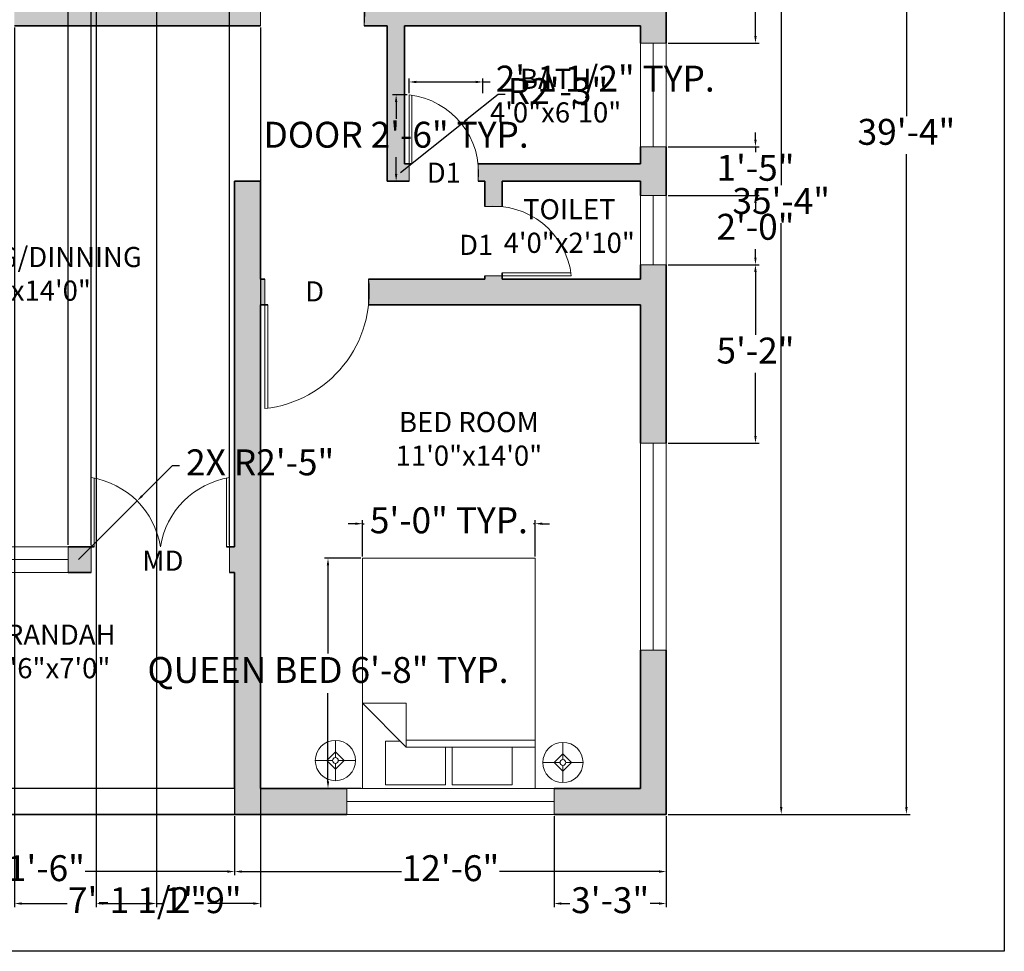
# Model space of a CAD drawing. Units: inches. Extents: x 1942 to 2601, y 2026 to 2623.
# Tile 4 of 5: x 2259 to 2601, y 2026 to 2350. Entities that reach past the tile are written whole.
import ezdxf

# ---------------------------------------------------------------- set-up
doc = ezdxf.new("R2010")
doc.units = ezdxf.units.IN
for name, color, linetype, lineweight in [('A-ANNO-DIMS', 2, 'Continuous', 18), ('A-ANNO-TEXT', 7, 'Continuous', 18), ('A-ANNO-TTLB', 7, 'Continuous', 25), ('A-AREA-IDEN', 7, 'Continuous', 25), ('A-DOOR', 4, 'Continuous', 18), ('A-FLOR', 7, 'Continuous', 25), ('A-FURN', 8, 'Continuous', 18), ('A-GLAZ', 2, 'Continuous', 18), ('A-WALL', 7, 'Continuous', 35), ('A-WALL-PATT', 7, 'Continuous', 13)]:
    doc.layers.add(name, color=color, linetype=linetype, lineweight=lineweight)
doc.styles.get("Standard").update_dxf_attribs({"font": 'arial.ttf'})
doc.dimstyles.new('ISO-25', dxfattribs={"dimtxt": 9, "dimasz": 2.5, "dimexe": 1.25, "dimexo": 0.625, "dimgap": 2, "dimtad": 0, "dimtih": 1, "dimtoh": 1, "dimdec": 1, "dimlunit": 4, "dimtxsty": 'Standard', "dimcen": 2.5, "dimadec": 0, "dimazin": 0, "dimtfac": 0.5, "dimtdec": 1, "dimtmove": 0, "dimatfit": 3, "dimfxl": 1, "dimarcsym": 0})

# ---------------------------------------------------------------- blocks, each defined once
blk = doc.blocks.new('Bed - Queen')
for p, q in [((0, -80.00003), (0, 0)), ((0, 0), (59.99999, 0)), ((59.99999, 0), (59.99999, -80.00003)), ((7.99999, -1.2), (28.79998, -1.2)), ((7.99999, -14.4), (7.99999, -1.2)), ((28.79998, -1.2), (28.79998, -14.4)), ((31.19999, -1.2), (51.99999, -1.2)), ((31.19999, -14.4), (31.19999, -1.2)), ((51.99999, -1.2), (51.99999, -16.4)), ((0, -14.4), (44.8, -14.4)), ((44.8, -16.8), (0, -16.8)), ((59.99999, -29.6), (44.8, -14.4)), ((44.8, -14.4), (44.8, -29.6)), ((51.99999, -16.4), (46.79936, -16.4)), ((44.8, -29.6), (59.99999, -29.6)), ((59.99999, -80.00003), (0, -80.00003))]:
    blk.add_line(p, q)
blk = doc.blocks.new('Lamp - Table')
for p, q in [((0, 7), (0, 1)), ((-1, 0), (-7, 0)), ((0, 3), (-3, 0)), ((-3, 0), (0, -3)), ((3, 0), (0, 3)), ((0, -3), (3, 0)), ((1, 0), (7, 0)), ((0, -1), (0, -7))]:
    blk.add_line(p, q)
for radius in [7, 1]:
    blk.add_circle((0, 0), radius)
blk = doc.blocks.new('*D21')
at = {"layer": 'A-ANNO-DIMS', "color": 0, "lineweight": -2, "transparency": 16777216}
for p, q in [((2195.82, 2073.29), (2195.82, 2052.78)), ((2333.82, 2073.29), (2333.82, 2052.78)), ((2198.32, 2054.03), (2247.78, 2054.03)), ((2331.32, 2054.03), (2281.85, 2054.03))]:
    blk.add_line(p, q, dxfattribs=at)
at = {"layer": 'A-ANNO-DIMS', "color": 0, "transparency": 16777216}
for points in [[(2198.32, 2054.45), (2198.32, 2053.61), (2195.82, 2054.03)], [(2331.32, 2054.45), (2331.32, 2053.61), (2333.82, 2054.03)]]:
    blk.add_solid(points, dxfattribs=at)
at = {"layer": 'Defpoints', "color": 0, "transparency": 16777216}
for p in [(2195.82, 2073.91), (2333.82, 2073.91), (2333.82, 2054.03)]:
    blk.add_point(p, dxfattribs=at)
at = {"layer": 'A-ANNO-DIMS', "color": 0, "transparency": 16777216, "insert": (2264.82, 2054.03), "char_height": 9, "attachment_point": 5}
blk.add_mtext('11\'-6"', dxfattribs=at)
blk = doc.blocks.new('*D22')
at = {"layer": 'A-ANNO-DIMS', "color": 0, "lineweight": -2, "transparency": 16777216}
for p, q in [((2333.82, 2073.29), (2333.82, 2052.78)), ((2483.82, 2073.29), (2483.82, 2052.78)), ((2336.32, 2054.03), (2391.78, 2054.03)), ((2481.32, 2054.03), (2425.85, 2054.03))]:
    blk.add_line(p, q, dxfattribs=at)
at = {"layer": 'A-ANNO-DIMS', "color": 0, "transparency": 16777216}
for points in [[(2336.32, 2054.45), (2336.32, 2053.61), (2333.82, 2054.03)], [(2481.32, 2054.45), (2481.32, 2053.61), (2483.82, 2054.03)]]:
    blk.add_solid(points, dxfattribs=at)
at = {"layer": 'Defpoints', "color": 0, "transparency": 16777216}
for p in [(2333.82, 2073.91), (2483.82, 2073.91), (2483.82, 2054.03)]:
    blk.add_point(p, dxfattribs=at)
at = {"layer": 'A-ANNO-DIMS', "color": 0, "transparency": 16777216, "insert": (2408.82, 2054.03), "char_height": 9, "attachment_point": 5}
blk.add_mtext('12\'-6"', dxfattribs=at)
blk = doc.blocks.new('*D23')
at = {"layer": 'A-ANNO-DIMS', "color": 0, "lineweight": -2, "transparency": 16777216}
for p, q in [((2484.44, 2497.91), (2525.02, 2497.91)), ((2523.77, 2495.41), (2523.77, 2292.51)), ((2523.77, 2076.41), (2523.77, 2279.32)), ((2484.44, 2073.91), (2525.02, 2073.91))]:
    blk.add_line(p, q, dxfattribs=at)
at = {"layer": 'A-ANNO-DIMS', "color": 0, "transparency": 16777216}
for points in [[(2523.35, 2495.41), (2524.19, 2495.41), (2523.77, 2497.91)], [(2523.35, 2076.41), (2524.19, 2076.41), (2523.77, 2073.91)]]:
    blk.add_solid(points, dxfattribs=at)
at = {"layer": 'Defpoints', "color": 0, "transparency": 16777216}
for p in [(2483.82, 2497.91), (2483.82, 2073.91), (2523.77, 2073.91)]:
    blk.add_point(p, dxfattribs=at)
at = {"layer": 'A-ANNO-DIMS', "color": 0, "transparency": 16777216, "insert": (2523.77, 2285.91), "char_height": 9, "attachment_point": 5}
blk.add_mtext('35\'-4"', dxfattribs=at)
blk = doc.blocks.new('*D24')
at = {"layer": 'A-ANNO-DIMS', "color": 0, "lineweight": -2, "transparency": 16777216}
for p, q in [((2484.44, 2545.91), (2568.53, 2545.91)), ((2567.28, 2543.41), (2567.28, 2316.51)), ((2567.28, 2076.41), (2567.28, 2303.32)), ((2484.44, 2073.91), (2568.53, 2073.91))]:
    blk.add_line(p, q, dxfattribs=at)
at = {"layer": 'A-ANNO-DIMS', "color": 0, "transparency": 16777216}
for points in [[(2566.86, 2543.41), (2567.7, 2543.41), (2567.28, 2545.91)], [(2566.86, 2076.41), (2567.7, 2076.41), (2567.28, 2073.91)]]:
    blk.add_solid(points, dxfattribs=at)
at = {"layer": 'Defpoints', "color": 0, "transparency": 16777216}
for p in [(2483.82, 2545.91), (2483.82, 2073.91), (2567.28, 2073.91)]:
    blk.add_point(p, dxfattribs=at)
at = {"layer": 'A-ANNO-DIMS', "color": 0, "transparency": 16777216, "insert": (2567.28, 2309.91), "char_height": 9, "attachment_point": 5}
blk.add_mtext('39\'-4"', dxfattribs=at)
blk = doc.blocks.new('WIN-72IN')
for p, q in [((0, 0), (0, 9)), ((0, 9), (72, 9)), ((72, 0), (72, 9)), ((0, 4.5), (72, 4.5)), ((0, 0), (72, 0))]:
    blk.add_line(p, q)
blk = doc.blocks.new('DOOR-SINGLE-36IN')
for p, q in [((0, 9), (0, 45)), ((1, 9), (1, 44.88)), ((0, 0), (0, 9)), ((36, 0), (36, 9))]:
    blk.add_line(p, q)
blk.add_arc((-4.5, 4.5), 40.75, 353.6598, 83.6598)
blk = doc.blocks.new('DOOR-SINGLE-24IN')
for p, q in [((0, 6), (0, 30)), ((1, 6), (1, 29.87)), ((0, 6), (0, 0)), ((24, 6), (24, 0))]:
    blk.add_line(p, q)
blk.add_arc((-3, 3), 27.17, 353.6598, 83.6598)
blk = doc.blocks.new('WIN-36IN')
for p, q in [((0, 36), (9, 36)), ((0, 36), (0, 0)), ((4.5, 36), (4.5, 0)), ((9, 36), (9, 0)), ((0, 0), (9, 0))]:
    blk.add_line(p, q)
blk = doc.blocks.new('*D37')
at = {"layer": 'A-ANNO-DIMS', "color": 0, "lineweight": -2, "transparency": 16777216}
for p, q in [((2393.83, 2323.91), (2388.7, 2323.91)), ((2389.95, 2321.41), (2389.95, 2315.57)), ((2389.95, 2296.41), (2389.95, 2302.26)), ((2393.83, 2293.91), (2388.7, 2293.91))]:
    blk.add_line(p, q, dxfattribs=at)
at = {"layer": 'A-ANNO-DIMS', "color": 0, "transparency": 16777216}
for points in [[(2389.53, 2321.41), (2390.37, 2321.41), (2389.95, 2323.91)], [(2389.53, 2296.41), (2390.37, 2296.41), (2389.95, 2293.91)]]:
    blk.add_solid(points, dxfattribs=at)
at = {"layer": 'Defpoints', "color": 0, "transparency": 16777216}
for p in [(2389.95, 2323.91), (2394.45, 2323.91), (2394.45, 2293.91)]:
    blk.add_point(p, dxfattribs=at)
at = {"layer": 'A-ANNO-DIMS', "color": 0, "transparency": 16777216, "insert": (2389.95, 2308.91), "char_height": 9, "attachment_point": 5}
blk.add_mtext('DOOR 2\'-6" TYP.', dxfattribs=at)
blk = doc.blocks.new('*D38')
at = {"layer": 'A-ANNO-DIMS', "color": 0, "lineweight": -2, "transparency": 16777216}
for p, q in [((2394.45, 2324.54), (2394.45, 2329.66)), ((2396.95, 2328.41), (2417.61, 2328.41)), ((2420.11, 2324.54), (2420.11, 2329.66)), ((2420.11, 2328.41), (2422.61, 2328.41))]:
    blk.add_line(p, q, dxfattribs=at)
at = {"layer": 'A-ANNO-DIMS', "color": 0, "transparency": 16777216}
for points in [[(2396.95, 2328.83), (2396.95, 2328), (2394.45, 2328.41)], [(2417.61, 2328.83), (2417.61, 2328), (2420.11, 2328.41)]]:
    blk.add_solid(points, dxfattribs=at)
at = {"layer": 'Defpoints', "color": 0, "transparency": 16777216}
for p in [(2420.11, 2328.41), (2394.45, 2323.91), (2420.11, 2323.91)]:
    blk.add_point(p, dxfattribs=at)
at = {"layer": 'A-ANNO-DIMS', "color": 0, "transparency": 16777216, "insert": (2462.6, 2328.41), "char_height": 9, "attachment_point": 5}
blk.add_mtext('2\'-1 1/2" TYP.', dxfattribs=at)
blk = doc.blocks.new('*D41')
at = {"layer": 'A-ANNO-DIMS', "color": 0, "lineweight": -2, "transparency": 16777216}
for p, q in [((2377.64, 2162.91), (2365.02, 2162.91)), ((2366.27, 2160.41), (2366.27, 2129.84)), ((2366.27, 2085.41), (2366.27, 2115.98)), ((2377.64, 2082.91), (2365.02, 2082.91))]:
    blk.add_line(p, q, dxfattribs=at)
at = {"layer": 'A-ANNO-DIMS', "color": 0, "transparency": 16777216}
for points in [[(2365.85, 2160.41), (2366.68, 2160.41), (2366.27, 2162.91)], [(2365.85, 2085.41), (2366.68, 2085.41), (2366.27, 2082.91)]]:
    blk.add_solid(points, dxfattribs=at)
at = {"layer": 'Defpoints', "color": 0, "transparency": 16777216}
for p in [(2378.27, 2162.91), (2366.27, 2082.91), (2378.27, 2082.91)]:
    blk.add_point(p, dxfattribs=at)
at = {"layer": 'A-ANNO-DIMS', "color": 0, "transparency": 16777216, "insert": (2366.27, 2122.91), "char_height": 9, "attachment_point": 5}
blk.add_mtext('QUEEN BED 6\'-8" TYP.', dxfattribs=at)
blk = doc.blocks.new('*D42')
at = {"layer": 'A-ANNO-DIMS', "color": 0, "lineweight": -2, "transparency": 16777216}
for p, q in [((2375.77, 2174.91), (2373.27, 2174.91)), ((2378.27, 2163.54), (2378.27, 2176.16)), ((2378.27, 2174.91), (2378.84, 2174.91)), ((2438.27, 2174.91), (2437.7, 2174.91)), ((2438.27, 2163.54), (2438.27, 2176.16)), ((2440.77, 2174.91), (2443.27, 2174.91))]:
    blk.add_line(p, q, dxfattribs=at)
at = {"layer": 'A-ANNO-DIMS', "color": 0, "transparency": 16777216}
for points in [[(2375.77, 2175.33), (2375.77, 2174.5), (2378.27, 2174.91)], [(2440.77, 2175.33), (2440.77, 2174.5), (2438.27, 2174.91)]]:
    blk.add_solid(points, dxfattribs=at)
at = {"layer": 'Defpoints', "color": 0, "transparency": 16777216}
for p in [(2378.27, 2174.91), (2378.27, 2162.91), (2438.27, 2162.91)]:
    blk.add_point(p, dxfattribs=at)
at = {"layer": 'A-ANNO-DIMS', "color": 0, "transparency": 16777216, "insert": (2408.27, 2174.91), "char_height": 9, "attachment_point": 5}
blk.add_mtext('5\'-0" TYP.', dxfattribs=at)
blk = doc.blocks.new('*D61')
at = {"layer": 'A-ANNO-DIMS', "color": 0, "lineweight": -2, "transparency": 16777216}
for p, q in [((2484.44, 2386.91), (2516.07, 2386.91)), ((2514.82, 2384.41), (2514.82, 2371.01)), ((2514.82, 2344.41), (2514.82, 2357.82)), ((2484.44, 2341.91), (2516.07, 2341.91))]:
    blk.add_line(p, q, dxfattribs=at)
at = {"layer": 'A-ANNO-DIMS', "color": 0, "transparency": 16777216}
for points in [[(2514.4, 2384.41), (2515.24, 2384.41), (2514.82, 2386.91)], [(2514.4, 2344.41), (2515.24, 2344.41), (2514.82, 2341.91)]]:
    blk.add_solid(points, dxfattribs=at)
at = {"layer": 'Defpoints', "color": 0, "transparency": 16777216}
for p in [(2483.82, 2386.91), (2483.82, 2341.91), (2514.82, 2341.91)]:
    blk.add_point(p, dxfattribs=at)
at = {"layer": 'A-ANNO-DIMS', "color": 0, "transparency": 16777216, "insert": (2514.82, 2364.41), "char_height": 9, "attachment_point": 5}
blk.add_mtext('3\'-9"', dxfattribs=at)
blk = doc.blocks.new('*D62')
at = {"layer": 'A-ANNO-DIMS', "color": 0, "lineweight": -2, "transparency": 16777216}
for p, q in [((2514.82, 2308.41), (2514.82, 2310.91)), ((2484.44, 2305.91), (2516.07, 2305.91)), ((2514.82, 2305.91), (2514.82, 2304.01)), ((2514.82, 2288.91), (2514.82, 2290.82)), ((2484.44, 2288.91), (2516.07, 2288.91)), ((2514.82, 2286.41), (2514.82, 2283.91))]:
    blk.add_line(p, q, dxfattribs=at)
at = {"layer": 'A-ANNO-DIMS', "color": 0, "transparency": 16777216}
for points in [[(2514.4, 2308.41), (2515.24, 2308.41), (2514.82, 2305.91)], [(2514.4, 2286.41), (2515.24, 2286.41), (2514.82, 2288.91)]]:
    blk.add_solid(points, dxfattribs=at)
at = {"layer": 'Defpoints', "color": 0, "transparency": 16777216}
for p in [(2483.82, 2305.91), (2483.82, 2288.91), (2514.82, 2288.91)]:
    blk.add_point(p, dxfattribs=at)
at = {"layer": 'A-ANNO-DIMS', "color": 0, "transparency": 16777216, "insert": (2514.82, 2297.41), "char_height": 9, "attachment_point": 5}
blk.add_mtext('1\'-5"', dxfattribs=at)
blk = doc.blocks.new('*D63')
at = {"layer": 'A-ANNO-DIMS', "color": 0, "lineweight": -2, "transparency": 16777216}
for p, q in [((2484.44, 2288.91), (2516.07, 2288.91)), ((2514.82, 2286.41), (2514.82, 2283.51)), ((2514.82, 2267.41), (2514.82, 2270.32)), ((2484.44, 2264.91), (2516.07, 2264.91))]:
    blk.add_line(p, q, dxfattribs=at)
at = {"layer": 'A-ANNO-DIMS', "color": 0, "transparency": 16777216}
for points in [[(2514.4, 2286.41), (2515.24, 2286.41), (2514.82, 2288.91)], [(2514.4, 2267.41), (2515.24, 2267.41), (2514.82, 2264.91)]]:
    blk.add_solid(points, dxfattribs=at)
at = {"layer": 'Defpoints', "color": 0, "transparency": 16777216}
for p in [(2483.82, 2288.91), (2483.82, 2264.91), (2514.82, 2264.91)]:
    blk.add_point(p, dxfattribs=at)
at = {"layer": 'A-ANNO-DIMS', "color": 0, "transparency": 16777216, "insert": (2514.82, 2276.91), "char_height": 9, "attachment_point": 5}
blk.add_mtext('2\'-0"', dxfattribs=at)
blk = doc.blocks.new('*D64')
at = {"layer": 'A-ANNO-DIMS', "color": 0, "lineweight": -2, "transparency": 16777216}
for p, q in [((2484.44, 2264.91), (2516.07, 2264.91)), ((2514.82, 2262.41), (2514.82, 2240.51)), ((2514.82, 2205.41), (2514.82, 2227.32)), ((2484.44, 2202.91), (2516.07, 2202.91))]:
    blk.add_line(p, q, dxfattribs=at)
at = {"layer": 'A-ANNO-DIMS', "color": 0, "transparency": 16777216}
for points in [[(2514.4, 2262.41), (2515.24, 2262.41), (2514.82, 2264.91)], [(2514.4, 2205.41), (2515.24, 2205.41), (2514.82, 2202.91)]]:
    blk.add_solid(points, dxfattribs=at)
at = {"layer": 'Defpoints', "color": 0, "transparency": 16777216}
for p in [(2483.82, 2264.91), (2483.82, 2202.91), (2514.82, 2202.91)]:
    blk.add_point(p, dxfattribs=at)
at = {"layer": 'A-ANNO-DIMS', "color": 0, "transparency": 16777216, "insert": (2514.82, 2233.91), "char_height": 9, "attachment_point": 5}
blk.add_mtext('5\'-2"', dxfattribs=at)
blk = doc.blocks.new('*D65')
at = {"layer": 'A-ANNO-DIMS', "color": 0, "lineweight": -2, "transparency": 16777216}
for p, q in [((2444.82, 2073.29), (2444.82, 2041.66)), ((2483.82, 2073.29), (2483.82, 2041.66)), ((2447.32, 2042.91), (2450.36, 2042.91)), ((2481.32, 2042.91), (2478.28, 2042.91))]:
    blk.add_line(p, q, dxfattribs=at)
at = {"layer": 'A-ANNO-DIMS', "color": 0, "transparency": 16777216}
for points in [[(2447.32, 2043.33), (2447.32, 2042.5), (2444.82, 2042.91)], [(2481.32, 2043.33), (2481.32, 2042.5), (2483.82, 2042.91)]]:
    blk.add_solid(points, dxfattribs=at)
at = {"layer": 'Defpoints', "color": 0, "transparency": 16777216}
for p in [(2444.82, 2073.91), (2483.82, 2073.91), (2483.82, 2042.91)]:
    blk.add_point(p, dxfattribs=at)
at = {"layer": 'A-ANNO-DIMS', "color": 0, "transparency": 16777216, "insert": (2464.32, 2042.91), "char_height": 9, "attachment_point": 5}
blk.add_mtext('3\'-3"', dxfattribs=at)
blk = doc.blocks.new('*D67')
at = {"layer": 'A-ANNO-DIMS', "color": 0, "lineweight": -2, "transparency": 16777216}
for p, q in [((2275.92, 2167.54), (2275.92, 2580.37)), ((2284.02, 2167.54), (2284.02, 2580.37)), ((2273.42, 2579.12), (2270.92, 2579.12)), ((2275.92, 2579.12), (2284.02, 2579.12)), ((2286.52, 2579.12), (2289.02, 2579.12))]:
    blk.add_line(p, q, dxfattribs=at)
at = {"layer": 'A-ANNO-DIMS', "color": 0, "transparency": 16777216}
for points in [[(2273.42, 2579.54), (2273.42, 2578.7), (2275.92, 2579.12)], [(2286.52, 2579.54), (2286.52, 2578.7), (2284.02, 2579.12)]]:
    blk.add_solid(points, dxfattribs=at)
at = {"layer": 'Defpoints', "color": 0, "transparency": 16777216}
for p in [(2284.02, 2579.12), (2275.92, 2166.91), (2284.02, 2166.91)]:
    blk.add_point(p, dxfattribs=at)
at = {"layer": 'A-ANNO-DIMS', "color": 0, "transparency": 16777216, "insert": (2302.98, 2579.12), "char_height": 9, "attachment_point": 5}
blk.add_mtext('0\'-8"', dxfattribs=at)
blk = doc.blocks.new('*D68')
at = {"layer": 'A-ANNO-DIMS', "color": 0, "lineweight": -2, "transparency": 16777216}
for p, q in [((2284.02, 2167.54), (2284.02, 2580.37)), ((2332.02, 2167.54), (2332.02, 2580.37)), ((2286.52, 2579.12), (2293.88, 2579.12)), ((2329.52, 2579.12), (2322.16, 2579.12))]:
    blk.add_line(p, q, dxfattribs=at)
at = {"layer": 'A-ANNO-DIMS', "color": 0, "transparency": 16777216}
for points in [[(2286.52, 2579.54), (2286.52, 2578.7), (2284.02, 2579.12)], [(2329.52, 2579.54), (2329.52, 2578.7), (2332.02, 2579.12)]]:
    blk.add_solid(points, dxfattribs=at)
at = {"layer": 'Defpoints', "color": 0, "transparency": 16777216}
for p in [(2332.02, 2579.12), (2284.02, 2166.91), (2332.02, 2166.91)]:
    blk.add_point(p, dxfattribs=at)
at = {"layer": 'A-ANNO-DIMS', "color": 0, "transparency": 16777216, "insert": (2308.02, 2579.12), "char_height": 9, "attachment_point": 5}
blk.add_mtext('4\'-0"', dxfattribs=at)
blk = doc.blocks.new('*D69')
at = {"layer": 'A-ANNO-DIMS', "color": 0, "lineweight": -2, "transparency": 16777216}
for p, q in [((2257.32, 2347.29), (2257.32, 2041.66)), ((2342.82, 2347.29), (2342.82, 2041.66)), ((2259.82, 2042.91), (2275.66, 2042.91)), ((2340.32, 2042.91), (2324.48, 2042.91))]:
    blk.add_line(p, q, dxfattribs=at)
at = {"layer": 'A-ANNO-DIMS', "color": 0, "transparency": 16777216}
for points in [[(2259.82, 2043.33), (2259.82, 2042.5), (2257.32, 2042.91)], [(2340.32, 2043.33), (2340.32, 2042.5), (2342.82, 2042.91)]]:
    blk.add_solid(points, dxfattribs=at)
at = {"layer": 'Defpoints', "color": 0, "transparency": 16777216}
for p in [(2257.32, 2347.91), (2342.82, 2347.91), (2342.82, 2042.91)]:
    blk.add_point(p, dxfattribs=at)
at = {"layer": 'A-ANNO-DIMS', "color": 0, "transparency": 16777216, "insert": (2300.07, 2042.91), "char_height": 9, "attachment_point": 5}
blk.add_mtext('7\'-1 1/2"', dxfattribs=at)
blk = doc.blocks.new('*D75')
at = {"layer": 'A-ANNO-DIMS', "color": 0, "lineweight": -2, "transparency": 16777216}
for p, q in [((2285.65, 2487.5), (2285.65, 2041.66)), ((2306.65, 2487.5), (2306.65, 2041.66)), ((2288.15, 2042.91), (2304.15, 2042.91)), ((2306.65, 2042.91), (2309.15, 2042.91))]:
    blk.add_line(p, q, dxfattribs=at)
at = {"layer": 'A-ANNO-DIMS', "color": 0, "transparency": 16777216}
for points in [[(2288.15, 2043.33), (2288.15, 2042.5), (2285.65, 2042.91)], [(2304.15, 2043.33), (2304.15, 2042.5), (2306.65, 2042.91)]]:
    blk.add_solid(points, dxfattribs=at)
at = {"layer": 'Defpoints', "color": 0, "transparency": 16777216}
for p in [(2285.65, 2488.12), (2306.65, 2488.12), (2306.65, 2042.91)]:
    blk.add_point(p, dxfattribs=at)
at = {"layer": 'A-ANNO-DIMS', "color": 0, "transparency": 16777216, "insert": (2322.69, 2042.91), "char_height": 9, "attachment_point": 5}
blk.add_mtext('1\'-9"', dxfattribs=at)
blk = doc.blocks.new('*D79')
at = {"layer": 'A-ANNO-DIMS', "color": 0, "lineweight": -2, "transparency": 16777216}
for p, q in [((2312.16, 2195.06), (2301.69, 2184.58)), ((2314.66, 2195.06), (2312.16, 2195.06)), ((2279.52, 2162.41), (2299.92, 2182.82))]:
    blk.add_line(p, q, dxfattribs=at)
at = {"layer": 'A-ANNO-DIMS', "color": 0, "transparency": 16777216}
blk.add_solid([(2301.39, 2184.88), (2301.98, 2184.29), (2299.92, 2182.82)], dxfattribs=at)
at = {"layer": 'Defpoints', "color": 0, "transparency": 16777216}
for p in [(2299.92, 2182.82), (2279.52, 2162.41)]:
    blk.add_point(p, dxfattribs=at)
at = {"layer": 'A-ANNO-DIMS', "color": 0, "transparency": 16777216, "insert": (2342.68, 2195.06), "char_height": 9, "attachment_point": 5}
blk.add_mtext('2X R2\'-5"', dxfattribs=at)
blk = doc.blocks.new('*D80')
at = {"layer": 'A-ANNO-DIMS', "color": 0, "lineweight": -2, "transparency": 16777216}
for p, q in [((2425.39, 2324.07), (2414.62, 2315.45)), ((2427.89, 2324.07), (2425.39, 2324.07)), ((2391.45, 2296.91), (2412.66, 2313.88))]:
    blk.add_line(p, q, dxfattribs=at)
at = {"layer": 'A-ANNO-DIMS', "color": 0, "transparency": 16777216}
blk.add_solid([(2414.36, 2315.77), (2414.88, 2315.12), (2412.66, 2313.88)], dxfattribs=at)
at = {"layer": 'Defpoints', "color": 0, "transparency": 16777216}
for p in [(2412.66, 2313.88), (2391.45, 2296.91)]:
    blk.add_point(p, dxfattribs=at)
at = {"layer": 'A-ANNO-DIMS', "color": 0, "transparency": 16777216, "insert": (2446.16, 2324.07), "char_height": 9, "attachment_point": 5}
blk.add_mtext('R2\'-3"', dxfattribs=at)

msp = doc.modelspace()

# ---------------------------------------------------------------- hatches: boundary and pattern name
at = {"layer": 'A-WALL-PATT'}
h = msp.add_hatch(color=256, dxfattribs=at)
h.dxf.hatch_style = 1
h.paths.add_polyline_path([(2056.54, 2497.91), (1999.82, 2497.91), (1999.82, 2347.91), (2008.82, 2347.91), (2028.82, 2347.91), (2028.82, 2356.91), (2008.82, 2356.91), (2008.82, 2488.91), (2056.54, 2488.91)])
h.paths.add_polyline_path([(2173.82, 2356.91), (2164.82, 2356.91), (2076.82, 2356.91), (2076.82, 2347.91), (2096.82, 2347.91), (2105.82, 2347.91), (2164.82, 2347.91), (2173.82, 2347.91)])
h.paths.add_polyline_path([(2173.82, 2488.91), (2173.82, 2497.91), (2173.82, 2536.91), (2179.57, 2536.91), (2179.57, 2545.91), (2173.82, 2545.91), (2164.82, 2545.91), (2164.82, 2497.91), (2161.07, 2497.91), (2161.07, 2488.91), (2164.82, 2488.91), (2164.82, 2392.91), (2173.82, 2392.91)])
h.paths.add_polyline_path([(2125.07, 2497.91), (2116.54, 2497.91), (2116.54, 2488.91), (2125.07, 2488.91, -0.055385)])
h.paths.add_polyline_path([(2266.32, 2545.91), (2257.32, 2545.91), (2251.57, 2545.91), (2251.57, 2536.91), (2257.32, 2536.91), (2257.32, 2497.91), (2257.32, 2488.91), (2257.32, 2347.91), (2318.82, 2347.91), (2342.82, 2347.91), (2342.82, 2356.91), (2318.82, 2356.91), (2318.82, 2386.91), (2314.32, 2386.91), (2314.32, 2356.91), (2266.32, 2356.91), (2266.32, 2410.91), (2289.34, 2410.91, -0.055385), (2289.34, 2416.91), (2266.32, 2416.91), (2266.32, 2488.91), (2278.32, 2488.91), (2278.32, 2497.91), (2266.32, 2497.91)])
h.paths.add_polyline_path([(2360.82, 2497.91), (2314.32, 2497.91), (2314.32, 2488.91), (2314.32, 2416.91), (2314.32, 2410.91), (2318.82, 2410.91), (2318.82, 2488.91), (2360.82, 2488.91)])
h.paths.add_polyline_path([(2483.82, 2497.91), (2432.82, 2497.91), (2432.82, 2488.91), (2474.82, 2488.91), (2474.82, 2458.91), (2483.82, 2458.91)])
h.paths.add_polyline_path([(2483.82, 2386.91), (2474.82, 2386.91), (2474.82, 2356.91), (2378.82, 2356.91, -0.055385), (2378.82, 2347.91), (2386.82, 2347.91), (2386.82, 2299.91), (2386.82, 2293.91), (2394.45, 2293.91), (2394.45, 2299.91), (2392.82, 2299.91), (2392.82, 2347.91), (2474.82, 2347.91), (2474.82, 2341.91), (2483.82, 2341.91)])
h.paths.add_polyline_path([(2483.82, 2305.91), (2474.82, 2305.91), (2474.82, 2299.91), (2418.45, 2299.91, -0.055385), (2418.45, 2293.91), (2420.82, 2293.91), (2420.82, 2285.08, -0.055385), (2426.82, 2285.08), (2426.82, 2293.91), (2474.82, 2293.91), (2474.82, 2288.91), (2483.82, 2288.91)])
h = msp.add_hatch(color=256, dxfattribs=at)
h.dxf.hatch_style = 1
h.paths.add_polyline_path([(2483.82, 2264.91), (2474.82, 2264.91), (2474.82, 2259.91), (2426.82, 2259.91), (2426.82, 2261.08), (2420.82, 2261.08), (2420.82, 2259.91), (2380.37, 2259.91, -0.055385), (2380.37, 2250.91), (2474.82, 2250.91), (2474.82, 2202.91), (2483.82, 2202.91)])
h.paths.add_polyline_path([(2483.82, 2130.91), (2474.82, 2130.91), (2474.82, 2082.91), (2444.82, 2082.91), (2444.82, 2073.91), (2483.82, 2073.91)])
h.paths.add_polyline_path([(2372.82, 2082.91), (2342.82, 2082.91), (2342.82, 2250.91), (2344.37, 2250.91), (2344.37, 2259.91), (2342.82, 2259.91), (2342.82, 2293.91), (2333.82, 2293.91), (2333.82, 2259.91), (2333.82, 2250.91), (2333.82, 2166.91), (2332.02, 2166.91), (2332.02, 2157.91), (2333.82, 2157.91), (2333.82, 2082.91), (2333.82, 2073.91), (2372.82, 2073.91)])
h.paths.add_polyline_path([(2204.82, 2091.91), (2195.82, 2091.91), (2195.82, 2082.91), (2204.82, 2082.91)])
h.paths.add_polyline_path([(2284.02, 2166.91), (2275.92, 2166.91), (2275.92, 2157.91), (2284.02, 2157.91)])
h.paths.add_polyline_path([(2203.92, 2166.91), (2195.82, 2166.91), (2105.82, 2166.91), (2096.82, 2166.91), (2096.82, 2157.91), (2105.82, 2157.91), (2195.82, 2157.91), (2203.92, 2157.91)])
h.paths.add_polyline_path([(2105.82, 2275.91), (2096.82, 2275.91), (2096.82, 2250.91), (2096.82, 2238.91), (2105.82, 2238.91), (2105.82, 2250.91)])

# ---------------------------------------------------------------- linework, layer by layer
at = {"layer": 'A-ANNO-TTLB'}
msp.add_lwpolyline([(1941.67, 2623.37), (2601.3, 2623.37), (2601.3, 2026.31), (1941.67, 2026.31)], close=True, dxfattribs=at)
at = {"layer": 'A-DOOR'}
for p, q in [((2284.02, 2166.91), (2284.02, 2190.91)), ((2285.02, 2166.91), (2285.02, 2190.74)), ((2331.02, 2166.91), (2331.02, 2190.74)), ((2332.02, 2166.91), (2332.02, 2190.91)), ((2284.02, 2157.91), (2284.02, 2166.91)), ((2332.02, 2157.91), (2332.02, 2166.91))]:
    msp.add_line(p, q, dxfattribs=at)
for centre, start, end in [((2279.52, 2162.41), 8.9726, 81.0274), ((2336.52, 2162.41), 98.9726, 171.0274)]:
    msp.add_arc(centre, 28.85, start, end, dxfattribs=at)
at = {"layer": 'A-FLOR'}
for q in [(2195.82, 2082.91), (2333.82, 2073.91)]:
    msp.add_line((2333.82, 2082.91), q, dxfattribs=at)
at = {"layer": 'A-GLAZ'}
for p, q in [((2474.82, 2288.91), (2483.82, 2288.91)), ((2474.82, 2288.91), (2474.82, 2264.91)), ((2479.32, 2288.91), (2479.32, 2264.91)), ((2483.82, 2288.91), (2483.82, 2264.91)), ((2474.82, 2264.91), (2483.82, 2264.91))]:
    msp.add_line(p, q, dxfattribs=at)
at = {"layer": 'A-WALL'}
for p, q in [((2483.82, 2386.91), (2483.82, 2341.91)), ((2318.82, 2347.91), (2257.32, 2347.91)), ((2318.82, 2347.91), (2342.82, 2347.91)), ((2378.82, 2347.91), (2386.82, 2347.91)), ((2386.82, 2347.91), (2386.82, 2299.91)), ((2392.82, 2347.91), (2392.82, 2299.91)), ((2392.82, 2347.91), (2474.82, 2347.91)), ((2474.82, 2347.91), (2474.82, 2341.91)), ((2474.82, 2305.91), (2474.82, 2299.91)), ((2483.82, 2305.91), (2483.82, 2288.91)), ((2386.82, 2299.91), (2386.82, 2293.91)), ((2392.82, 2299.91), (2395.45, 2299.91)), ((2418.45, 2299.91), (2474.82, 2299.91)), ((2342.82, 2293.91), (2333.82, 2293.91)), ((2333.82, 2259.91), (2333.82, 2293.91)), ((2342.82, 2259.91), (2342.82, 2293.91)), ((2386.82, 2293.91), (2394.45, 2293.91)), ((2418.45, 2293.91), (2420.82, 2293.91)), ((2420.82, 2293.91), (2420.82, 2285.08)), ((2426.82, 2293.91), (2426.82, 2285.08)), ((2426.82, 2293.91), (2474.82, 2293.91)), ((2474.82, 2293.91), (2474.82, 2288.91)), ((2426.82, 2262.08), (2426.82, 2259.91)), ((2474.82, 2264.91), (2474.82, 2259.91)), ((2483.82, 2264.91), (2483.82, 2202.91)), ((2333.82, 2250.91), (2333.82, 2259.91)), ((2344.37, 2259.91), (2342.82, 2259.91)), ((2420.82, 2259.91), (2380.37, 2259.91)), ((2420.82, 2261.08), (2420.82, 2259.91)), ((2474.82, 2259.91), (2426.82, 2259.91)), ((2333.82, 2250.91), (2333.82, 2166.91)), ((2342.82, 2250.91), (2342.82, 2082.91)), ((2345.37, 2250.91), (2342.82, 2250.91)), ((2474.82, 2250.91), (2380.37, 2250.91)), ((2474.82, 2250.91), (2474.82, 2202.91)), ((2285.02, 2166.91), (2275.92, 2166.91)), ((2333.82, 2166.91), (2331.02, 2166.91)), ((2284.02, 2157.91), (2275.92, 2157.91)), ((2333.82, 2157.91), (2332.02, 2157.91)), ((2333.82, 2157.91), (2333.82, 2082.91)), ((2474.82, 2130.91), (2474.82, 2082.91)), ((2483.82, 2130.91), (2483.82, 2073.91)), ((2372.82, 2082.91), (2342.82, 2082.91)), ((2474.82, 2082.91), (2444.82, 2082.91)), ((2372.82, 2073.91), (2195.82, 2073.91)), ((2483.82, 2073.91), (2444.82, 2073.91))]:
    msp.add_line(p, q, dxfattribs=at)

# ---------------------------------------------------------------- block references
at = {"layer": 'A-DOOR'}
for name, p in [('DOOR-SINGLE-36IN', (2342.82, 2347.91)), ('DOOR-SINGLE-24IN', (2394.45, 2293.91))]:
    msp.add_blockref(name, p, dxfattribs=at)
at = {"layer": 'A-DOOR', "extrusion": (0, 0, -1), "zscale": -1}
for name, p, rotation in [('DOOR-SINGLE-24IN', (-2420.82, 2261.08), 90.00000000000088), ('DOOR-SINGLE-36IN', (-2344.37, 2259.91), 180)]:
    msp.add_blockref(name, p, dxfattribs=dict(at, rotation=rotation))
at = {"layer": 'A-FURN', "rotation": 180}
msp.add_blockref('Bed - Queen', (2438.27, 2082.91), dxfattribs=at)
at = {"layer": 'A-FURN'}
for p in [(2368.85, 2092.61), (2447.91, 2091.92)]:
    msp.add_blockref('Lamp - Table', p, dxfattribs=at)
at = {"layer": 'A-GLAZ'}
msp.add_blockref('WIN-36IN', (2474.82, 2305.91), dxfattribs=at)
for p, rotation in [((2474.82, 2202.91), 269.9999999999995), ((2275.92, 2166.91), 180), ((2444.82, 2082.91), 180)]:
    msp.add_blockref('WIN-72IN', p, dxfattribs=dict(at, rotation=rotation))

# ---------------------------------------------------------------- texts
at = {"layer": 'A-ANNO-TEXT', "char_height": 7, "attachment_point": 1}
for s, width, insert in [('\\pxqc;D1', 19.5389, (2396.77, 2300.37)), ('\\pxqc;D1', 19.5389, (2407.99, 2275.3)), ('\\pxqc;D', 19.5389, (2351.86, 2259.13)), ('\\pxqc;MD', 13.9054, (2301.93, 2165.56))]:
    msp.add_mtext_dynamic_manual_height_columns(s, width=width, gutter_width=12.5, heights=[0], dxfattribs=dict(at, insert=insert))
at = {"layer": 'A-AREA-IDEN', "char_height": 7, "attachment_point": 1}
for s, width, insert in [('\\pxqc;{\\fArial|b1|i0|c0|p34;BATH\\P4\'0"x6\'10"}', 49.35, (2420.71, 2333)), ('\\pxqc;{\\fArial|b1|i0|c0|p34;TOILET\\P4\'0"x2\'10}"', 40.6886, (2429.77, 2287.69)), ('\\pxqc;{\\fArial|b1|i0|c0|p34;DRAWING/DINNING\\P19\'0"x14\'0"}', 128.6303, (2194.11, 2271.08)), ('\\pxqc;{\\fArial|b1|i0|c0|p34;BED ROOM\\P11\'0"x14\'0"}', 95.2426, (2367.63, 2213.73)), ('\\pxqc;{\\fArial|b1|i0|c0|p34;VERANDAH\\P11\'6"x7\'0"}', 112.3172, (2211.67, 2139.87))]:
    msp.add_mtext_dynamic_manual_height_columns(s, width=width, gutter_width=12.5, heights=[0], dxfattribs=dict(at, insert=insert))

# ---------------------------------------------------------------- dimensions: what is measured, and where the dimension line sits
at = {"layer": 'A-ANNO-DIMS'}
for base, p1, p2, override, picture, middle in [((2284.02, 2579.12), (2275.92, 2166.91), (2284.02, 2166.91), {"dimdec": 1, "dimlfac": 1, "dimrnd": 0, "dimzin": 1, "dimdsep": 46, "dimlunit": 4, "dimfrac": 2}, '*D67', (2302.98, 2579.12)), ((2332.02, 2579.12), (2284.02, 2166.91), (2332.02, 2166.91), {"dimdec": 1, "dimlfac": 1, "dimrnd": 0, "dimzin": 1, "dimdsep": 46, "dimlunit": 4, "dimfrac": 2}, '*D68', (2308.02, 2579.12)), ((2306.65, 2042.91), (2285.65, 2488.12), (2306.65, 2488.12), {"dimdec": 1, "dimlfac": 1, "dimrnd": 0, "dimzin": 1, "dimdsep": 46, "dimlunit": 4, "dimfrac": 2}, '*D75', (2322.69, 2042.91)), ((2342.82, 2042.91), (2257.32, 2347.91), (2342.82, 2347.91), {"dimdec": 1, "dimlfac": 1, "dimrnd": 0, "dimzin": 1, "dimdsep": 46, "dimlunit": 4, "dimfrac": 2}, '*D69', (2300.07, 2042.91)), ((2333.82, 2054.03), (2195.82, 2073.91), (2333.82, 2073.91), {"dimclrd": 0, "dimclre": 0, "dimclrt": 0}, '*D21', (2264.82, 2054.03)), ((2483.82, 2054.03), (2333.82, 2073.91), (2483.82, 2073.91), {"dimclrd": 0, "dimclre": 0, "dimclrt": 0}, '*D22', (2408.82, 2054.03)), ((2483.82, 2042.91), (2444.82, 2073.91), (2483.82, 2073.91), {"dimdec": 1, "dimlfac": 1, "dimrnd": 0, "dimzin": 1, "dimdsep": 46, "dimlunit": 4, "dimfrac": 2}, '*D65', (2464.32, 2042.91))]:
    dim = msp.add_linear_dim(base=base, p1=p1, p2=p2, dimstyle='ISO-25', override=override, dxfattribs=at)
    dim.commit()
    dim.dimension.update_dxf_attribs({"geometry": picture, "text_midpoint": middle})
for base, p1, p2, override, picture, middle in [((2567.28, 2073.91), (2483.82, 2545.91), (2483.82, 2073.91), {"dimclrd": 0, "dimclre": 0, "dimclrt": 0}, '*D24', (2567.28, 2309.91)), ((2523.77, 2073.91), (2483.82, 2497.91), (2483.82, 2073.91), {"dimclrd": 0, "dimclre": 0, "dimclrt": 0}, '*D23', (2523.77, 2285.91)), ((2514.82, 2341.91), (2483.82, 2386.91), (2483.82, 2341.91), {"dimdec": 1, "dimlfac": 1, "dimrnd": 0, "dimzin": 1, "dimdsep": 46, "dimlunit": 4, "dimfrac": 2}, '*D61', (2514.82, 2364.41)), ((2514.82, 2288.91), (2483.82, 2305.91), (2483.82, 2288.91), {"dimdec": 1, "dimlfac": 1, "dimrnd": 0, "dimzin": 1, "dimdsep": 46, "dimlunit": 4, "dimfrac": 2}, '*D62', (2514.82, 2297.41)), ((2514.82, 2264.91), (2483.82, 2288.91), (2483.82, 2264.91), {"dimdec": 1, "dimlfac": 1, "dimrnd": 0, "dimzin": 1, "dimdsep": 46, "dimlunit": 4, "dimfrac": 2}, '*D63', (2514.82, 2276.91)), ((2514.82, 2202.91), (2483.82, 2264.91), (2483.82, 2202.91), {"dimdec": 1, "dimlfac": 1, "dimrnd": 0, "dimzin": 1, "dimdsep": 46, "dimlunit": 4, "dimfrac": 2}, '*D64', (2514.82, 2233.91))]:
    dim = msp.add_linear_dim(base=base, p1=p1, p2=p2, angle=90, dimstyle='ISO-25', override=override, dxfattribs=at)
    dim.commit()
    dim.dimension.update_dxf_attribs({"geometry": picture, "text_midpoint": middle})
dim = msp.add_linear_dim(base=(2420.11, 2328.41), p1=(2394.45, 2323.91), p2=(2420.11, 2323.91), text='<> TYP.', dimstyle='ISO-25', override={"dimdec": 1, "dimlfac": 1, "dimrnd": 0, "dimzin": 1, "dimdsep": 46, "dimlunit": 4, "dimfrac": 2}, dxfattribs=at)
dim.commit()
dim.dimension.update_dxf_attribs({"geometry": '*D38', "text_midpoint": (2462.6, 2328.41)})
dim = msp.add_radius_dim(center=(2391.45, 2296.91), mpoint=(2412.66, 2313.88), dimstyle='ISO-25', override={"dimdec": 1, "dimlfac": 1, "dimrnd": 0, "dimzin": 1, "dimdsep": 46, "dimlunit": 4, "dimfrac": 2}, dxfattribs=at)
dim.commit()
dim.dimension.update_dxf_attribs({"geometry": '*D80', "text_midpoint": (2446.16, 2324.07), "dimtype": 164})
for base, p1, p2, angle, text, picture, middle in [((2389.95, 2323.91), (2394.45, 2293.91), (2394.45, 2323.91), 90, 'DOOR <> TYP.', '*D37', (2389.95, 2308.91)), ((2378.27, 2174.91), (2438.27, 2162.91), (2378.27, 2162.91), 180, '<> TYP.', '*D42', (2408.27, 2174.91)), ((2366.27, 2082.91), (2378.27, 2162.91), (2378.27, 2082.91), 270, 'QUEEN BED <> TYP.', '*D41', (2366.27, 2122.91))]:
    dim = msp.add_linear_dim(base=base, p1=p1, p2=p2, angle=angle, text=text, dimstyle='ISO-25', override={"dimdec": 1, "dimlfac": 1, "dimrnd": 0, "dimzin": 1, "dimdsep": 46, "dimlunit": 4, "dimfrac": 2}, dxfattribs=at)
    dim.commit()
    dim.dimension.update_dxf_attribs({"geometry": picture, "text_midpoint": middle})
dim = msp.add_radius_dim(center=(2279.52, 2162.41), mpoint=(2299.92, 2182.82), text='2X <>', dimstyle='ISO-25', override={"dimdec": 1, "dimlfac": 1, "dimrnd": 0, "dimzin": 1, "dimdsep": 46, "dimlunit": 4, "dimfrac": 2}, dxfattribs=at)
dim.commit()
dim.dimension.update_dxf_attribs({"geometry": '*D79', "text_midpoint": (2342.68, 2195.06), "dimtype": 164})

doc.saveas('drawing.dxf')
